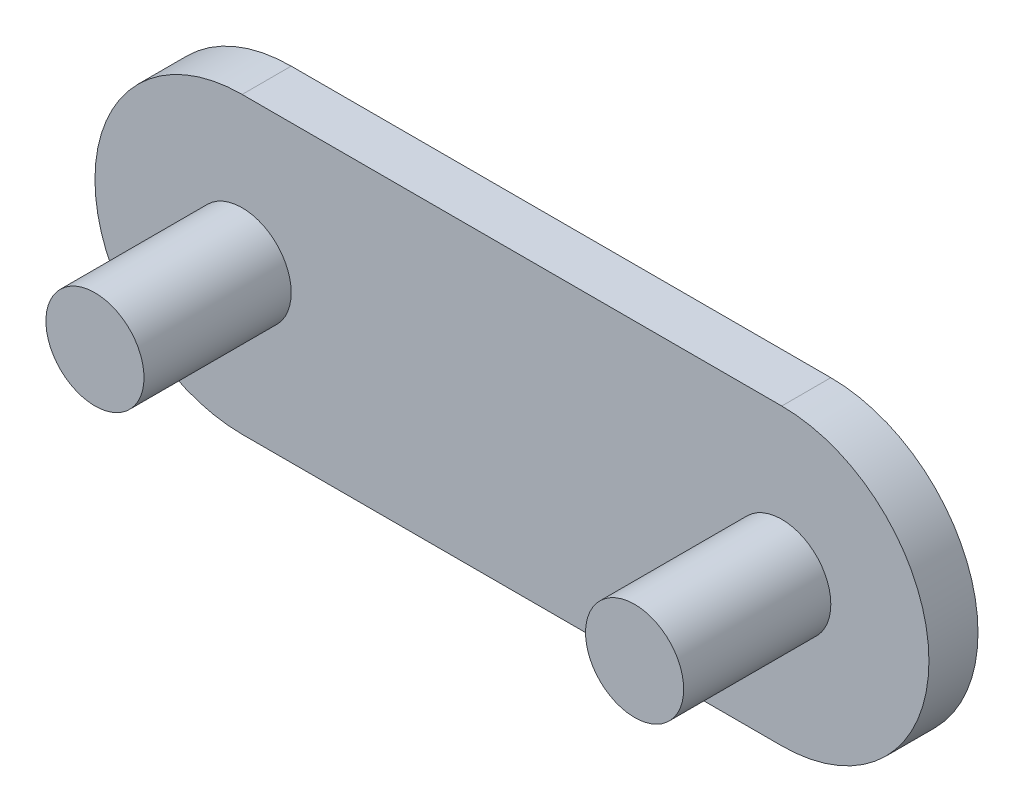
from build123d import *

# Parameters (mm, degrees)
LINK_PLATE_DEPTH = 5
SKETCH1_3_R      = 5
PINS_2X_10_DEPTH = 15


with BuildPart() as part:
    # Link Profile Sketch → Link Plate (new body)
    with BuildSketch(Plane.XY):
        with BuildLine():
            Line((27.5, -15), (-27.5, -15))
            ThreePointArc((-27.5, -15), (-42.5, 0), (-27.5, 15))
            Line((-27.5, 15), (27.5, 15))
            ThreePointArc((27.5, 15), (42.5, 0), (27.5, -15))
        make_face()
    extrude(amount=-LINK_PLATE_DEPTH)

    # Sketch1_3 → Pins 2x_10 (add)
    with BuildSketch(Plane.XY):
        with Locations((-27.5, 0)):
            Circle(SKETCH1_3_R)
        with Locations((27.5, 0)):
            Circle(SKETCH1_3_R)
    extrude(amount=PINS_2X_10_DEPTH)


solid = part.part
